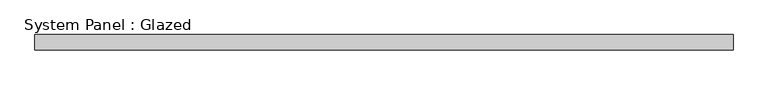
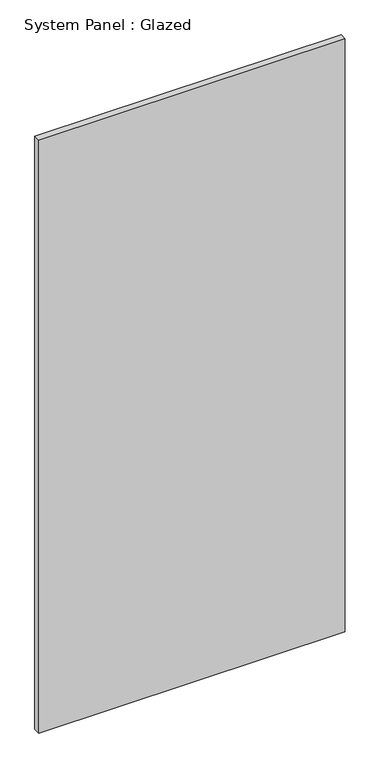
"""IFC4 building model written with IfcOpenShell, lengths in millimetres: plate geometry, System Panel : Glazed."""

from ifc_helpers import new_model, si_unit, origin, origin_with_axes, place, context, project, spatial, polyline, outline, extrude, source, transform, mapped, element, save


def system_panel_glazed_3787533d(model_context):
    return source(origin(), model_context, "Body", "SweptSolid", [
        extrude(outline(polyline([(572.1, 24.5), (-572.1, 24.5), (-572.1, 49.5), (572.1, 49.5), (572.1, 24.5)])), origin_with_axes(), (0.0, 0.0, 1.0), 2338.4),
    ])


if __name__ == "__main__":
    model = new_model("IFC4")
    model_context = context("Model", 3, world=origin())
    ifc_project = project(units=[si_unit("LENGTHUNIT", "METRE", prefix="MILLI")], contexts=[model_context])
    site = spatial("IfcSite", under=ifc_project)
    building = spatial("IfcBuilding", under=site)
    placement = place(None, origin())
    system_panel_glazed_shape = system_panel_glazed_3787533d(model_context)
    element("IfcPlate", 1, ObjectType="System Panel : Glazed", at=placement, inside=building, context=model_context, shape_type="MappedRepresentation", body=[
        mapped(system_panel_glazed_shape, transform((0.0, 0.0, 0.0), x_axis=(1.0, 0.0, 0.0), y_axis=(0.0, 1.0, 0.0), z_axis=(0.0, 0.0, 1.0))),
    ])
    save(model, "model.ifc")

# Revit data of these elements
# Type "System Panel : Glazed"
#   Construction Type Id = "GSP4R"
#   Analytic Construction = "1/8 in Pilkington single glazing"
#   Visual Light Transmittance = 0.9
#   Solar Heat Gain Coefficient = 0.86
#   Heat Transfer Coefficient (U) = 6.7069 W/(m²·K)
# Element 1 (IfcPlate, "System Panel : Glazed")
#   Materials on its faces: "Glass"
# Materials
#   "Glass": class "Glass", colour RGB 0 128 192, transparency 0.9, Description = "Soda Lime Glass", Cost = 0
